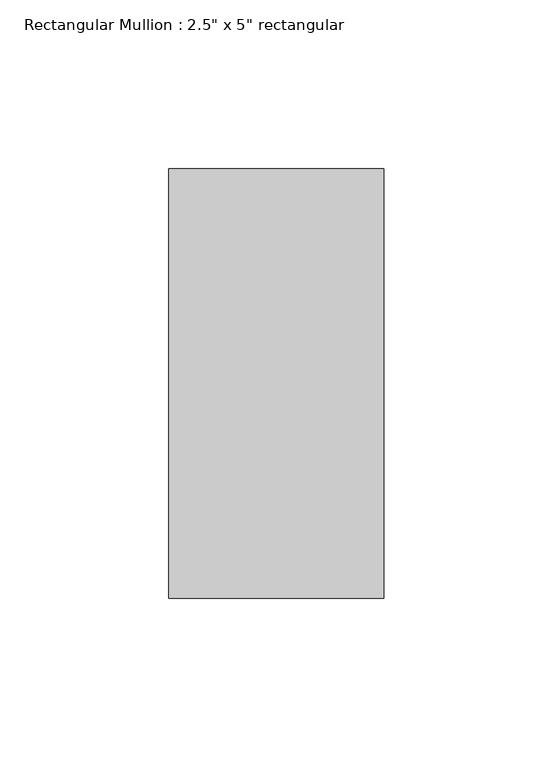
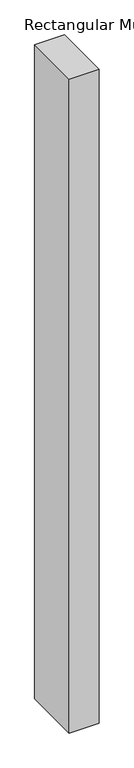
"""IFC4 building model written with IfcOpenShell, lengths in millimetres: member geometry."""

from ifc_helpers import new_model, si_unit, frame, origin, place, context, project, spatial, polyline, outline, extrude, source, transform, mapped, element, save


def member_6e88ea55(model_context):
    return source(origin(), model_context, "Body", "SweptSolid", [
        extrude(outline(polyline([(31.75, 63.5), (31.75, -63.5), (-31.75, -63.5), (-31.75, 63.5), (31.75, 63.5)])), frame((0.0, 0.0, -1472.0504916), z_axis=(0.0, 0.0, 1.0), x_axis=(1.0, 0.0, 0.0)), (0.0, 0.0, 1.0), 1472.0504916),
    ])


if __name__ == "__main__":
    model = new_model("IFC4")
    model_context = context("Model", 3, world=origin())
    ifc_project = project(units=[si_unit("LENGTHUNIT", "METRE", prefix="MILLI")], contexts=[model_context])
    site = spatial("IfcSite", under=ifc_project)
    building = spatial("IfcBuilding", under=site)
    placement = place(None, origin())
    member_shape = member_6e88ea55(model_context)
    element("IfcMember", 1, ObjectType="Rectangular Mullion : 2.5\" x 5\" rectangular", at=placement, inside=building, context=model_context, shape_type="MappedRepresentation", body=[
        mapped(member_shape, transform((0.0, 0.0, 0.0), x_axis=(1.0, 0.0, 0.0), y_axis=(0.0, 1.0, 0.0), z_axis=(0.0, 0.0, 1.0))),
    ])
    save(model, "model.ifc")

# Revit data of these elements
# Type "Rectangular Mullion : 2.5\" x 5\" rectangular"
#   built-in parameter 1007304 = 0.416667 (stored number, unit not read)
#   built-in parameter 1007301 = 0.104167 (stored number, unit not read)
#   built-in parameter 1007300 = 0.104167 (stored number, unit not read)
# Element 1 (IfcMember, "Rectangular Mullion : 2.5\" x 5\" rectangular")
#   Materials on its faces: "Aluminum"
# Materials
#   "Aluminum": class "Metal", colour RGB 247 247 247, transparency 0, Description = "Aluminum 6061", Cost = 0
